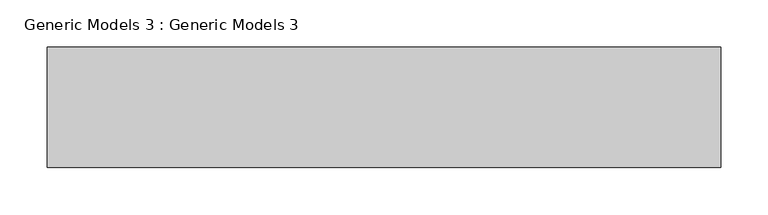
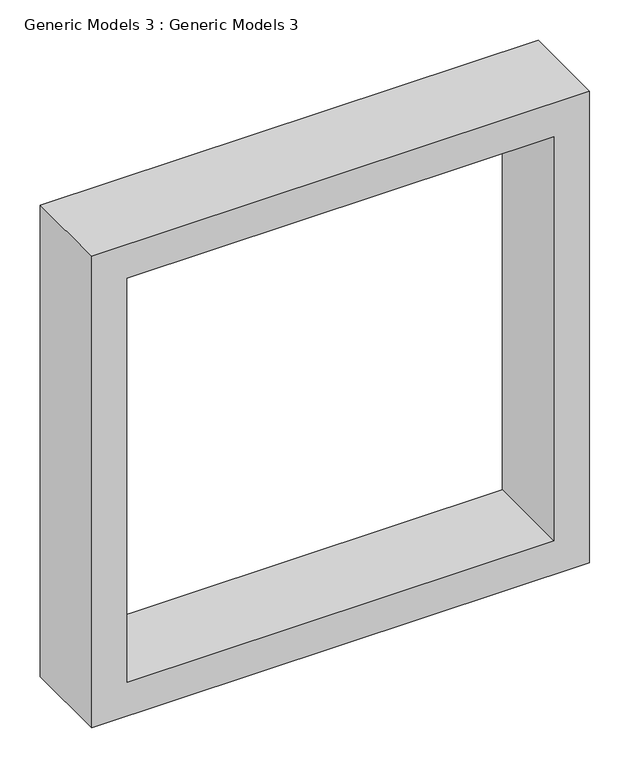
"""IFC4 building model written with IfcOpenShell, lengths in millimetres: proxy geometry, Generic Models 3 : Generic Models 3."""

from ifc_helpers import new_model, si_unit, frame, origin, place, context, project, spatial, polyline, outline, extrude, source, transform, mapped, element, save


def generic_models_3_generic_models_3_ef4d42f5(model_context):
    return source(origin(), model_context, "Body", "SweptSolid", [
        extrude(outline(polyline([(6146.8, -5721.373248), (6146.8, -6432.573248), (5435.6, -6432.573248), (5435.6, -5721.373248), (6146.8, -5721.373248)]), holes=[polyline([(6096.0, -5772.173248), (5486.4, -5772.173248), (5486.4, -6381.773248), (6096.0, -6381.773248), (6096.0, -5772.173248)])]), frame((0.0, -3899.4866303, 0.0), z_axis=(0.0, 1.0, 0.0), x_axis=(0.0, 0.0, 1.0)), (0.0, 0.0, 1.0), 127.0),
    ])


if __name__ == "__main__":
    model = new_model("IFC4")
    model_context = context("Model", 3, world=origin())
    ifc_project = project(units=[si_unit("LENGTHUNIT", "METRE", prefix="MILLI")], contexts=[model_context])
    site = spatial("IfcSite", under=ifc_project)
    building = spatial("IfcBuilding", under=site)
    placement = place(None, origin())
    generic_models_3_generic_models_3_shape = generic_models_3_generic_models_3_ef4d42f5(model_context)
    element("IfcBuildingElementProxy", 1, Name="Generic Models 3 : Generic Models 3", ObjectType="Generic Models 3 : Generic Models 3", at=placement, inside=building, context=model_context, shape_type="MappedRepresentation", body=[
        mapped(generic_models_3_generic_models_3_shape, transform((0.0, 0.0, 0.0), x_axis=(1.0, 0.0, 0.0), y_axis=(0.0, 1.0, 0.0), z_axis=(0.0, 0.0, 1.0))),
    ])
    save(model, "model.ifc")

# Revit data of these elements
# Element 1 (IfcBuildingElementProxy, "Generic Models 3 : Generic Models 3")
#   Materials on its faces: "BLACK FRAMING 6\""
# Materials
#   "BLACK FRAMING 6\"": class "Generic", colour RGB 120 120 120, transparency 0, Cost = 0
